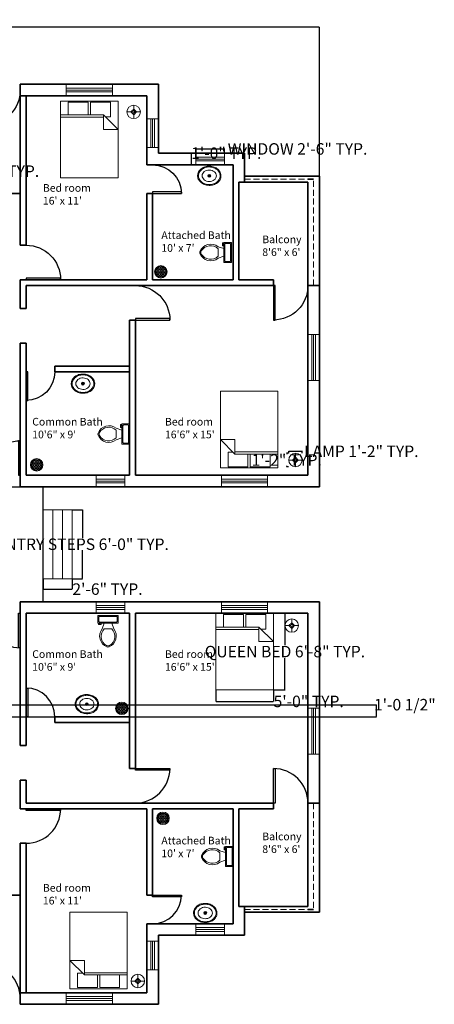
# Model space of a CAD drawing. Units: inches. Extents: x 2450 to 4494, y 1482 to 2597.
# Tile 7 of 7: x 4062 to 4494, y 1559 to 2587. Entities that reach past the tile are written whole.
import ezdxf

# ---------------------------------------------------------------- set-up
doc = ezdxf.new("R2010")
doc.units = ezdxf.units.IN
doc.header["$LTSCALE"] = 5
doc.header["$MEASUREMENT"] = 0
doc.linetypes.add('HIDDEN', pattern=[0.375, 0.25, -0.125])
for name, color, linetype, lineweight in [('A-ANNO-DIMS', 2, 'Continuous', 18), ('A-AREA-IDEN', 7, 'Continuous', 18), ('A-DOOR', 4, 'Continuous', 25), ('A-FLOR-EDGE', 7, 'Continuous', 25), ('A-FLOR-FIXT', 9, 'Continuous', 18), ('A-FLOR-STRS', 7, 'Continuous', 18), ('A-FURN', 8, 'Continuous', 18), ('A-GLAZ', 4, 'Continuous', 18), ('A-WALL', 7, 'Continuous', 35), ('A-WALL-HIDN', 7, 'HIDDEN', 18)]:
    doc.layers.add(name, color=color, linetype=linetype, lineweight=lineweight)
doc.styles.get("Standard").update_dxf_attribs({"font": 'arial.ttf'})
doc.dimstyles.get("Standard").update_dxf_attribs({"dimtxt": 12, "dimasz": 0.18, "dimexe": 0.18, "dimexo": 0.0625, "dimgap": 0.09, "dimtad": 0, "dimtih": 1, "dimtoh": 1, "dimdec": 0, "dimzin": 0, "dimdsep": 46, "dimlunit": 3, "dimtxsty": 'Standard', "dimcen": 0.09, "dimadec": 0, "dimazin": 0, "dimtfac": 1, "dimtdec": 0, "dimtofl": 0, "dimtmove": 0, "dimatfit": 3, "dimfxl": 1, "dimtolj": 1, "dimtzin": 0, "dimarcsym": 0})

# ---------------------------------------------------------------- blocks, each defined once
blk = doc.blocks.new('*U2')
for p, q in [((0, 0), (0, -6)), ((36, 0), (36, -6))]:
    blk.add_line(p, q)
blk.add_lwpolyline([(0, 0), (0, 36), (1.75, 36), (1.75, 0)], close=True)
blk.add_arc((0, 0), 36, 0, 90)
blk = doc.blocks.new('*U3')
for p, q in [((0, 0), (0, -6)), ((30, 0), (30, -6))]:
    blk.add_line(p, q)
blk.add_lwpolyline([(0, 0), (0, 30), (1.75, 30), (1.75, 0)], close=True)
blk.add_arc((0, 0), 30, 0, 90)
blk = doc.blocks.new('*U5')
for p, q in [((-36, 0), (-36, 6)), ((0, 0), (0, 6))]:
    blk.add_line(p, q)
blk.add_lwpolyline([(0, 0), (0, -36), (-1.75, -36), (-1.75, 0)], close=True)
blk.add_arc((0, 0), 36, 180, 270)
blk = doc.blocks.new('Bed - Queen')
for p, q in [((0, -80.00003), (0, 0)), ((0, 0), (59.99999, 0)), ((59.99999, 0), (59.99999, -80.00003)), ((7.99999, -1.2), (28.79998, -1.2)), ((7.99999, -14.4), (7.99999, -1.2)), ((28.79998, -1.2), (28.79998, -14.4)), ((31.19999, -1.2), (51.99999, -1.2)), ((31.19999, -14.4), (31.19999, -1.2)), ((51.99999, -1.2), (51.99999, -16.4)), ((0, -14.4), (44.8, -14.4)), ((44.8, -16.8), (0, -16.8)), ((59.99999, -29.6), (44.8, -14.4)), ((44.8, -14.4), (44.8, -29.6)), ((51.99999, -16.4), (46.79936, -16.4)), ((44.8, -29.6), (59.99999, -29.6)), ((59.99999, -80.00003), (0, -80.00003))]:
    blk.add_line(p, q)
blk = doc.blocks.new('Lamp - Table')
for p, q in [((-1, 0), (-7, 0)), ((0, 3), (-3, 0)), ((-3, 0), (0, -3)), ((0, 7), (0, 1)), ((3, 0), (0, 3)), ((0, -3), (3, 0)), ((1, 0), (7, 0)), ((0, -1), (0, -7))]:
    blk.add_line(p, q)
for radius in [7, 1]:
    blk.add_circle((0, 0), radius)
blk = doc.blocks.new('Toilet - top')
for p, q in [((-10, -8.5), (-8, -8.5)), ((-10, -9.5), (-10, -8.5)), ((-7, -9.5), (-10, -9.5)), ((-8, -8.5), (-8, -8)), ((-7, -8), (-7, -9.5)), ((-4, -8), (-6, -14)), ((4, -8), (6, -14)), ((9.5, -6), (9.5, -2)), ((4, -14), (-4, -14))]:
    blk.add_line(p, q)
blk.add_lwpolyline([(10.5, -8), (10.5, 0), (-10.5, 0), (-10.5, -8)], close=True)
for points in [[(-9.5, -2), (-9.5, -6)], [(8.5, -1), (-8.5, -1)], [(-8.5, -7), (8.5, -7)]]:
    blk.add_lwpolyline(points)
for centre, radius, start, end in [((-8.6, -1.9), 0.884, 81.8699, 188.1301), ((-8.6, -6.1), 0.884, 171.8699, 278.1301), ((8.6, -1.9), 0.884, 351.8699, 98.1301), ((8.6, -6.1), 0.884, 261.8699, 8.1301), ((3.5, -21.6), 12.2, 141.4691, 247.9714), ((4.2, -21.8), 11.3, 136.3677, 238.9468), ((-3.5, -21.6), 12.2, 292.0284, 38.5307), ((-4.2, -21.8), 11.3, 301.053, 43.6321), ((0, -27.9), 4, 245.7318, 294.2682), ((0, -29), 4, 254.8605, 285.1395)]:
    blk.add_arc(centre, radius, start, end)
blk = doc.blocks.new('Sink - Oval top')
for p, q in [((-1, 0), (1, 0)), ((0, 1), (0, -1))]:
    blk.add_line(p, q)
for points in [[(-12.2, 0.4, 0.117634), (-11.5, -3.4, 0.104469), (-8.9, -6.8, 0.090016), (-5.1, -9.1, 0.08192), (-0.3, -10, 0.08192), (4.5, -9.4, 0.090016), (8.4, -7.4, 0.104469), (11.2, -4.1, 0.117634), (12.2, -0.4, 0.117634), (11.5, 3.4, 0.104469), (8.9, 6.8, 0.090016), (5.1, 9.1, 0.08192), (0.3, 10, 0.08192), (-4.5, 9.4, 0.090016), (-8.4, 7.4, 0.104469), (-11.2, 4.1, 0.117634)], [(-11.3, 0.2, 0.118622), (-10.5, -3.3, 0.104678), (-8.1, -6.4, 0.089562), (-4.5, -8.4, 0.081185), (-0.1, -9.2, 0.081185), (4.3, -8.5, 0.089562), (7.9, -6.6, 0.104678), (10.4, -3.5, 0.118622), (11.3, -0.2, 0.118622), (10.5, 3.3, 0.104678), (8.1, 6.4, 0.089562), (4.5, 8.4, 0.081185), (0.1, 9.2, 0.081185), (-4.3, 8.5, 0.089562), (-7.9, 6.6, 0.104678), (-10.4, 3.5, 0.118622)], [(-7.4, 0.1, 0.118283), (-6.9, -2.2, 0.104607), (-5.3, -4.2, 0.089718), (-3, -5.5, 0.081436), (-0.1, -6, 0.081436), (2.8, -5.6, 0.089718), (5.2, -4.3, 0.104607), (6.9, -2.3, 0.118283), (7.4, -0.1, 0.118283), (6.9, 2.2, 0.104607), (5.3, 4.2, 0.089718), (3, 5.5, 0.081436), (0.1, 6, 0.081436), (-2.8, 5.6, 0.089718), (-5.2, 4.3, 0.104607), (-6.9, 2.3, 0.118283)]]:
    blk.add_lwpolyline(points, format="xyb", close=True)
for radius in [1.5, 1]:
    blk.add_circle((0, 0), radius)
blk = doc.blocks.new('WIN-30-FRAME')
for p, q in [((0, 0), (0, 12)), ((0, 12), (30, 12)), ((30, 12), (30, 0)), ((30, 8), (0, 8)), ((30, 6), (0, 6)), ((30, 4), (0, 4)), ((30, 0), (0, 0))]:
    blk.add_line(p, q)
blk = doc.blocks.new('WIN-48-FRAME')
for p, q in [((48, 12), (0, 12)), ((0, 12), (0, 0)), ((48, 0), (48, 12)), ((48, 8), (0, 8)), ((48, 6), (0, 6)), ((48, 4), (0, 4)), ((0, 0), (48, 0))]:
    blk.add_line(p, q)
blk = doc.blocks.new('WIN-30-PART-FRAME')
for p, q in [((12, 30), (0, 30)), ((0, 30), (0, 0)), ((4, 30), (4, 0)), ((6, 30), (6, 0)), ((8, 30), (8, 0)), ((12, 6), (12, 30)), ((0, 0), (12, 0))]:
    blk.add_line(p, q)
blk = doc.blocks.new('WIN-48-PART-FRAME')
for p, q in [((48, 12), (0, 12)), ((0, 12), (0, 0)), ((48, 0), (48, 12)), ((48, 8), (0, 8)), ((48, 6), (0, 6)), ((48, 4), (0, 4)), ((24, 0), (48, 0))]:
    blk.add_line(p, q)
blk = doc.blocks.new('WIN-48-OPEN-SIDE')
for p, q in [((0, 48), (12, 48)), ((4, 48), (4, 0)), ((6, 48), (6, 0)), ((8, 48), (8, 0)), ((12, 48), (12, 0)), ((12, 0), (0, 0))]:
    blk.add_line(p, q)
blk = doc.blocks.new('STEPS-72-ENTRY')
at = {"ltscale": 5}
for p, q in [((0, 72), (30, 72)), ((10, 0), (10, 72)), ((20, 0), (20, 72)), ((30, 0), (30, 72)), ((0, 0), (30, 0))]:
    blk.add_line(p, q, dxfattribs=at)
blk = doc.blocks.new('DRAIN-FLOOR-ROUND')
at = {"ltscale": 5}
h = blk.add_hatch(dxfattribs=at)
h.set_pattern_fill('HONEY', color=256, scale=7)
h.set_pattern_definition([(0, (-4161.689, -1861.538), (1.3125, 0.75777223), [0.875, -1.75]), (120, (-4161.689, -1861.538), (-1.3125, 0.75777223), [0.875, -1.75]), (60, (-4161.689, -1861.538), (3e-16, 1.51554446), [-1.75, 0.875])])
h.paths.add_polyline_path([(1, 6.5, 1), (12, 6.5, 1)])
for radius in [6.52, 5.52]:
    blk.add_circle((6.5, 6.5), radius, dxfattribs=at)
blk = doc.blocks.new('*D39')
at = {"layer": 'A-ANNO-DIMS', "color": 0, "lineweight": -2, "ltscale": 5, "transparency": 16777216}
for p, q in [((4245.3, 2447.3), (4245.3, 2451.9)), ((4245.5, 2451.8), (4275.1, 2451.8)), ((4275.3, 2447.3), (4275.3, 2451.9)), ((4275.3, 2451.8), (4275.5, 2451.8))]:
    blk.add_line(p, q, dxfattribs=at)
at = {"layer": 'A-ANNO-DIMS', "color": 0, "ltscale": 5, "transparency": 16777216}
for points in [[(4245.5, 2451.8), (4245.5, 2451.7), (4245.3, 2451.8)], [(4275.1, 2451.8), (4275.1, 2451.7), (4275.3, 2451.8)]]:
    blk.add_solid(points, dxfattribs=at)
at = {"layer": 'Defpoints', "color": 0, "ltscale": 5, "transparency": 16777216}
for p in [(4245.3, 2447.3), (4275.3, 2451.8), (4275.3, 2447.3)]:
    blk.add_point(p, dxfattribs=at)
at = {"layer": 'A-ANNO-DIMS', "color": 0, "ltscale": 5, "transparency": 16777216, "insert": (4351.5, 2451.8), "char_height": 12, "attachment_point": 5}
blk.add_mtext('\\A1;WINDOW 2\'-6" TYP.', dxfattribs=at)
blk = doc.blocks.new('*D40')
at = {"layer": 'A-ANNO-DIMS', "color": 0, "lineweight": -2, "ltscale": 5, "transparency": 16777216}
for p, q in [((4245.2, 2447.3), (4240.6, 2447.3)), ((4240.8, 2447.3), (4240.8, 2447.4)), ((4240.8, 2447.4), (4241, 2447.4)), ((4240.8, 2435.4), (4240.8, 2447.1)), ((4245.2, 2435.3), (4240.6, 2435.3))]:
    blk.add_line(p, q, dxfattribs=at)
at = {"layer": 'A-ANNO-DIMS', "color": 0, "ltscale": 5, "transparency": 16777216}
for points in [[(4240.8, 2447.1), (4240.8, 2447.1), (4240.8, 2447.3)], [(4240.8, 2435.4), (4240.8, 2435.4), (4240.8, 2435.3)]]:
    blk.add_solid(points, dxfattribs=at)
at = {"layer": 'Defpoints', "color": 0, "ltscale": 5, "transparency": 16777216}
for p in [(4240.8, 2447.3), (4245.3, 2447.3), (4245.3, 2435.3)]:
    blk.add_point(p, dxfattribs=at)
at = {"layer": 'A-ANNO-DIMS', "color": 0, "ltscale": 5, "transparency": 16777216, "insert": (4277.1, 2447.4), "char_height": 12, "attachment_point": 5}
blk.add_mtext('\\A1;1\'-0" TYP.', dxfattribs=at)
blk = doc.blocks.new('*D49')
at = {"layer": 'A-ANNO-DIMS', "color": 0, "lineweight": -2, "ltscale": 5, "transparency": 16777216}
for p, q in [((4326.4, 1967.3), (4338.5, 1967.3)), ((4338.3, 1967.1), (4338.3, 1933.9)), ((4338.3, 1887.4), (4338.3, 1920.6)), ((4326.4, 1887.3), (4338.5, 1887.3))]:
    blk.add_line(p, q, dxfattribs=at)
at = {"layer": 'A-ANNO-DIMS', "color": 0, "ltscale": 5, "transparency": 16777216}
for points in [[(4338.3, 1967.1), (4338.3, 1967.1), (4338.3, 1967.3)], [(4338.3, 1887.4), (4338.3, 1887.4), (4338.3, 1887.3)]]:
    blk.add_solid(points, dxfattribs=at)
at = {"layer": 'Defpoints', "color": 0, "ltscale": 5, "transparency": 16777216}
for p in [(4326.3, 1967.3), (4338.3, 1967.3), (4326.3, 1887.3)]:
    blk.add_point(p, dxfattribs=at)
at = {"layer": 'A-ANNO-DIMS', "color": 0, "ltscale": 5, "transparency": 16777216, "insert": (4338.3, 1927.3), "char_height": 12, "attachment_point": 5}
blk.add_mtext('\\A1;QUEEN BED 6\'-8" TYP.', dxfattribs=at)
blk = doc.blocks.new('*D50')
at = {"layer": 'A-ANNO-DIMS', "color": 0, "lineweight": -2, "ltscale": 5, "transparency": 16777216}
for p, q in [((4266.3, 1887.2), (4266.3, 1875.1)), ((4326.3, 1887.2), (4326.3, 1875.1)), ((4266.5, 1875.3), (4326.1, 1875.3)), ((4326.3, 1875.3), (4326.5, 1875.3))]:
    blk.add_line(p, q, dxfattribs=at)
at = {"layer": 'A-ANNO-DIMS', "color": 0, "ltscale": 5, "transparency": 16777216}
for points in [[(4266.5, 1875.3), (4266.5, 1875.2), (4266.3, 1875.3)], [(4326.1, 1875.3), (4326.1, 1875.2), (4326.3, 1875.3)]]:
    blk.add_solid(points, dxfattribs=at)
at = {"layer": 'Defpoints', "color": 0, "ltscale": 5, "transparency": 16777216}
for p in [(4266.3, 1887.3), (4326.3, 1887.3), (4326.3, 1875.3)]:
    blk.add_point(p, dxfattribs=at)
at = {"layer": 'A-ANNO-DIMS', "color": 0, "ltscale": 5, "transparency": 16777216, "insert": (4363.1, 1875.3), "char_height": 12, "attachment_point": 5}
blk.add_mtext('\\A1;5\'-0" TYP.', dxfattribs=at)
blk = doc.blocks.new('*D51')
at = {"layer": 'A-ANNO-DIMS', "color": 0, "lineweight": -2, "ltscale": 5, "transparency": 16777216}
for p, q in [((4342.3, 2134.2), (4342.3, 2136.5)), ((4342.5, 2136.3), (4356.1, 2136.3)), ((4356.3, 2134.2), (4356.3, 2136.5)), ((4356.3, 2136.3), (4356.5, 2136.3))]:
    blk.add_line(p, q, dxfattribs=at)
at = {"layer": 'A-ANNO-DIMS', "color": 0, "ltscale": 5, "transparency": 16777216}
for points in [[(4342.5, 2136.3), (4342.5, 2136.2), (4342.3, 2136.3)], [(4356.1, 2136.3), (4356.1, 2136.2), (4356.3, 2136.3)]]:
    blk.add_solid(points, dxfattribs=at)
at = {"layer": 'Defpoints', "color": 0, "ltscale": 5, "transparency": 16777216}
for p in [(4342.3, 2134.2), (4356.3, 2136.3), (4356.3, 2134.2)]:
    blk.add_point(p, dxfattribs=at)
at = {"layer": 'A-ANNO-DIMS', "color": 0, "ltscale": 5, "transparency": 16777216, "insert": (4418, 2136.3), "char_height": 12, "attachment_point": 5}
blk.add_mtext('\\A1;LAMP 1\'-2" TYP.', dxfattribs=at)
blk = doc.blocks.new('*D52')
at = {"layer": 'A-ANNO-DIMS', "color": 0, "lineweight": -2, "ltscale": 5, "transparency": 16777216}
for p, q in [((4342.2, 2134.2), (4340, 2134.2)), ((4340.2, 2134), (4340.2, 2133.3)), ((4342.2, 2120.2), (4340, 2120.2)), ((4340.2, 2120.4), (4340.2, 2121.1))]:
    blk.add_line(p, q, dxfattribs=at)
at = {"layer": 'A-ANNO-DIMS', "color": 0, "ltscale": 5, "transparency": 16777216}
for points in [[(4340.1, 2134), (4340.2, 2134), (4340.2, 2134.2)], [(4340.1, 2120.4), (4340.2, 2120.4), (4340.2, 2120.2)]]:
    blk.add_solid(points, dxfattribs=at)
at = {"layer": 'Defpoints', "color": 0, "ltscale": 5, "transparency": 16777216}
for p in [(4340.2, 2134.2), (4342.3, 2134.2), (4342.3, 2120.2)]:
    blk.add_point(p, dxfattribs=at)
at = {"layer": 'A-ANNO-DIMS', "color": 0, "ltscale": 5, "transparency": 16777216, "insert": (4340.2, 2127.2), "char_height": 12, "attachment_point": 5}
blk.add_mtext('\\A1;1\'-2" TYP.', dxfattribs=at)
blk = doc.blocks.new('*D65')
at = {"layer": 'A-ANNO-DIMS', "color": 0, "lineweight": -2, "ltscale": 5, "transparency": 16777216}
for p, q in [((4014, 2458.6), (4023.1, 2458.6)), ((4022.9, 2458.4), (4022.9, 2434.9)), ((4022.9, 2398.7), (4022.9, 2422.3)), ((4014, 2398.6), (4023.1, 2398.6))]:
    blk.add_line(p, q, dxfattribs=at)
at = {"layer": 'A-ANNO-DIMS', "color": 0, "ltscale": 5, "transparency": 16777216}
for points in [[(4022.9, 2458.4), (4022.9, 2458.4), (4022.9, 2458.6)], [(4022.9, 2398.7), (4022.9, 2398.7), (4022.9, 2398.6)]]:
    blk.add_solid(points, dxfattribs=at)
at = {"layer": 'Defpoints', "color": 0, "ltscale": 5, "transparency": 16777216}
for p in [(4013.9, 2458.6), (4022.9, 2458.6), (4013.9, 2398.6)]:
    blk.add_point(p, dxfattribs=at)
at = {"layer": 'A-ANNO-DIMS', "color": 0, "ltscale": 5, "transparency": 16777216, "insert": (4022.9, 2428.6), "char_height": 12, "attachment_point": 5}
blk.add_mtext('\\A1;DESK 5\'-0" TYP.', dxfattribs=at)
blk = doc.blocks.new('*D67')
at = {"layer": 'A-ANNO-DIMS', "color": 0, "lineweight": -2, "ltscale": 5, "transparency": 16777216}
for p, q in [((4116.4, 2075.3), (4127.3, 2075.3)), ((4127.1, 2075.1), (4127.1, 2045.6)), ((4127.1, 2003.4), (4127.1, 2033)), ((4116.4, 2003.3), (4127.3, 2003.3))]:
    blk.add_line(p, q, dxfattribs=at)
at = {"layer": 'A-ANNO-DIMS', "color": 0, "ltscale": 5, "transparency": 16777216}
for points in [[(4127.1, 2075.1), (4127.1, 2075.1), (4127.1, 2075.3)], [(4127.1, 2003.4), (4127.1, 2003.4), (4127.1, 2003.3)]]:
    blk.add_solid(points, dxfattribs=at)
at = {"layer": 'Defpoints', "color": 0, "ltscale": 5, "transparency": 16777216}
for p in [(4116.3, 2075.3), (4127.1, 2075.3), (4116.3, 2003.3)]:
    blk.add_point(p, dxfattribs=at)
at = {"layer": 'A-ANNO-DIMS', "color": 0, "ltscale": 5, "transparency": 16777216, "insert": (4127.1, 2039.3), "char_height": 12, "attachment_point": 5}
blk.add_mtext('\\A1;ENTRY STEPS 6\'-0" TYP.', dxfattribs=at)
blk = doc.blocks.new('*D68')
at = {"layer": 'A-ANNO-DIMS', "color": 0, "lineweight": -2, "ltscale": 5, "transparency": 16777216}
for p, q in [((4086.3, 2003.2), (4086.3, 1992.3)), ((4116.3, 2003.2), (4116.3, 1992.3)), ((4086.5, 1992.5), (4116.1, 1992.5)), ((4116.3, 1992.5), (4116.5, 1992.5))]:
    blk.add_line(p, q, dxfattribs=at)
at = {"layer": 'A-ANNO-DIMS', "color": 0, "ltscale": 5, "transparency": 16777216}
for points in [[(4086.5, 1992.5), (4086.5, 1992.4), (4086.3, 1992.5)], [(4116.1, 1992.5), (4116.1, 1992.4), (4116.3, 1992.5)]]:
    blk.add_solid(points, dxfattribs=at)
at = {"layer": 'Defpoints', "color": 0, "ltscale": 5, "transparency": 16777216}
for p in [(4086.3, 2003.3), (4116.3, 2003.3), (4116.3, 1992.5)]:
    blk.add_point(p, dxfattribs=at)
at = {"layer": 'A-ANNO-DIMS', "color": 0, "ltscale": 5, "transparency": 16777216, "insert": (4153.2, 1992.5), "char_height": 12, "attachment_point": 5}
blk.add_mtext('\\A1;2\'-6" TYP.', dxfattribs=at)
blk = doc.blocks.new('*D71')
at = {"layer": 'A-ANNO-DIMS', "color": 0, "lineweight": -2, "ltscale": 5, "transparency": 16777216}
for p, q in [((3258.3, 2423.3), (3258.3, 2578.9)), ((3258.5, 2578.8), (3795.6, 2578.8)), ((4374.1, 2578.8), (3837, 2578.8)), ((4374.3, 2423.3), (4374.3, 2578.9))]:
    blk.add_line(p, q, dxfattribs=at)
at = {"layer": 'A-ANNO-DIMS', "color": 0, "ltscale": 5, "transparency": 16777216}
for points in [[(3258.5, 2578.8), (3258.5, 2578.7), (3258.3, 2578.8)], [(4374.1, 2578.8), (4374.1, 2578.7), (4374.3, 2578.8)]]:
    blk.add_solid(points, dxfattribs=at)
at = {"layer": 'Defpoints', "color": 0, "ltscale": 5, "transparency": 16777216}
for p in [(4374.3, 2578.8), (3258.3, 2423.3), (4374.3, 2423.3)]:
    blk.add_point(p, dxfattribs=at)
at = {"layer": 'A-ANNO-DIMS', "color": 0, "ltscale": 5, "transparency": 16777216, "insert": (3816.3, 2578.8), "char_height": 12, "attachment_point": 5}
blk.add_mtext('\\A1;93\'-0"', dxfattribs=at)
blk = doc.blocks.new('*D87')
at = {"layer": 'A-ANNO-DIMS', "color": 0, "lineweight": -2, "ltscale": 5, "transparency": 16777216}
for p, q in [((3504.9, 1871.8), (4434, 1871.8)), ((4433.8, 1871.8), (4433.8, 1871.9)), ((4433.8, 1871.9), (4434, 1871.9)), ((4433.8, 1859.4), (4433.8, 1871.6)), ((3534.4, 1859.3), (4434, 1859.3))]:
    blk.add_line(p, q, dxfattribs=at)
at = {"layer": 'A-ANNO-DIMS', "color": 0, "ltscale": 5, "transparency": 16777216}
for points in [[(4433.8, 1871.6), (4433.8, 1871.6), (4433.8, 1871.8)], [(4433.8, 1859.4), (4433.8, 1859.4), (4433.8, 1859.3)]]:
    blk.add_solid(points, dxfattribs=at)
at = {"layer": 'Defpoints', "color": 0, "ltscale": 5, "transparency": 16777216}
for p in [(3504.9, 1871.8), (4433.8, 1871.8), (3534.3, 1859.3)]:
    blk.add_point(p, dxfattribs=at)
at = {"layer": 'A-ANNO-DIMS', "color": 0, "ltscale": 5, "transparency": 16777216, "insert": (4463.4, 1871.9), "char_height": 12, "attachment_point": 5}
blk.add_mtext('\\A1;1\'-0 1/2"', dxfattribs=at)

msp = doc.modelspace()

# ---------------------------------------------------------------- linework, layer by layer
at = {"layer": 'A-FLOR-EDGE', "ltscale": 5}
for p in [(3546.29, 2099.27), (4086.29, 1979.27)]:
    msp.add_line(p, (4086.29, 2099.27), dxfattribs=at)
at = {"layer": 'A-WALL'}
for p, q in [((4062.29, 2519.27), (4206.29, 2519.27)), ((4062.29, 2507.27), (4062.29, 2519.27)), ((4206.29, 2507.27), (4206.29, 2519.27)), ((4062.29, 2507.27), (4194.29, 2507.27)), ((4062.29, 2351.27), (4062.29, 2507.27)), ((4068.29, 2351.27), (4068.29, 2507.27)), ((4194.29, 2507.27), (4194.29, 2435.27)), ((4206.29, 2507.27), (4206.29, 2447.27)), ((4284.29, 2447.27), (4206.29, 2447.27)), ((4284.29, 2447.27), (4296.29, 2447.27)), ((4296.29, 2447.27), (4296.29, 2423.27)), ((4200.29, 2435.27), (4194.29, 2435.27)), ((4284.29, 2435.27), (4200.29, 2435.27)), ((4284.29, 2435.27), (4284.29, 2315.27)), ((4290.29, 2417.27), (4290.29, 2315.27)), ((4362.29, 2417.27), (4290.29, 2417.27)), ((4362.29, 2423.27), (4296.29, 2423.27)), ((4296.29, 2423.27), (4296.29, 2417.27)), ((4362.29, 2423.27), (4374.29, 2423.27)), ((4362.29, 2420.27), (4368.29, 2420.27)), ((4362.29, 2417.27), (4362.29, 2315.27)), ((4374.29, 2423.27), (4374.29, 2099.27)), ((4062.29, 2405.27), (3930.29, 2405.27)), ((4194.29, 2405.27), (4194.29, 2315.27)), ((4200.29, 2405.27), (4194.29, 2405.27)), ((4200.29, 2405.27), (4200.29, 2315.27)), ((4068.29, 2351.27), (4062.29, 2351.27)), ((4062.29, 2285.27), (4062.29, 2315.27)), ((4068.29, 2315.27), (4062.29, 2315.27)), ((4176.29, 2315.27), (4068.29, 2315.27)), ((4182.29, 2315.27), (4176.29, 2315.27)), ((4194.29, 2315.27), (4182.29, 2315.27)), ((4284.29, 2315.27), (4200.29, 2315.27)), ((4326.29, 2315.27), (4290.29, 2315.27)), ((4326.29, 2309.27), (4326.29, 2315.27)), ((4362.29, 2309.27), (4362.29, 2315.27)), ((4068.29, 2285.27), (4068.29, 2309.27)), ((4176.29, 2309.27), (4068.29, 2309.27)), ((4176.29, 2309.27), (4182.29, 2309.27)), ((4326.29, 2309.27), (4182.29, 2309.27)), ((4362.29, 2309.27), (4362.29, 2111.27)), ((4362.29, 2309.27), (4374.29, 2309.27)), ((4068.29, 2285.27), (4062.29, 2285.27)), ((4176.29, 2111.27), (4176.29, 2273.27)), ((4176.29, 2273.27), (4182.29, 2273.27)), ((4182.29, 2111.27), (4182.29, 2273.27)), ((4062.29, 2111.27), (4062.29, 2249.27)), ((4068.29, 2249.27), (4062.29, 2249.27)), ((4068.29, 2225.27), (4068.29, 2249.27)), ((4068.29, 2219.27), (4068.29, 2225.27)), ((4068.29, 2111.27), (4068.29, 2219.27)), ((4176.29, 2225.27), (4098.29, 2225.27)), ((4098.29, 2219.27), (4098.29, 2225.27)), ((4176.29, 2219.27), (4098.29, 2219.27)), ((4062.29, 2111.27), (4062.29, 2099.27)), ((4176.29, 2111.27), (4068.29, 2111.27)), ((4362.29, 2111.27), (4182.29, 2111.27)), ((4374.29, 2099.27), (4062.29, 2099.27)), ((4374.29, 1979.27), (4062.29, 1979.27)), ((4062.29, 1967.27), (4062.29, 1979.27)), ((4374.29, 1655.27), (4374.29, 1979.27)), ((4062.29, 1967.27), (4062.29, 1829.27)), ((4176.29, 1967.27), (4068.29, 1967.27)), ((4068.29, 1967.27), (4068.29, 1859.27)), ((4176.29, 1967.27), (4176.29, 1805.27)), ((4362.29, 1967.27), (4182.29, 1967.27)), ((4182.29, 1967.27), (4182.29, 1805.27)), ((4362.29, 1769.27), (4362.29, 1967.27)), ((4068.29, 1859.27), (4068.29, 1853.27)), ((4068.29, 1853.27), (4068.29, 1829.27)), ((4176.29, 1859.27), (4098.29, 1859.27)), ((4098.29, 1859.27), (4098.29, 1853.27)), ((4176.29, 1853.27), (4098.29, 1853.27)), ((4068.29, 1829.27), (4062.29, 1829.27)), ((4176.29, 1805.27), (4182.29, 1805.27)), ((4062.29, 1793.27), (4062.29, 1763.27)), ((4068.29, 1793.27), (4062.29, 1793.27)), ((4068.29, 1793.27), (4068.29, 1769.27)), ((4176.29, 1769.27), (4068.29, 1769.27)), ((4176.29, 1769.27), (4182.29, 1769.27)), ((4326.29, 1769.27), (4182.29, 1769.27)), ((4326.29, 1769.27), (4326.29, 1763.27)), ((4362.29, 1769.27), (4362.29, 1763.27)), ((4362.29, 1769.27), (4374.29, 1769.27)), ((4068.29, 1763.27), (4062.29, 1763.27)), ((4176.29, 1763.27), (4068.29, 1763.27)), ((4182.29, 1763.27), (4176.29, 1763.27)), ((4194.29, 1763.27), (4182.29, 1763.27)), ((4194.29, 1673.27), (4194.29, 1763.27)), ((4200.29, 1673.27), (4200.29, 1763.27)), ((4284.29, 1763.27), (4200.29, 1763.27)), ((4284.29, 1643.27), (4284.29, 1763.27)), ((4290.29, 1661.27), (4290.29, 1763.27)), ((4326.29, 1763.27), (4290.29, 1763.27)), ((4362.29, 1661.27), (4362.29, 1763.27)), ((4062.29, 1727.27), (4062.29, 1571.27)), ((4068.29, 1727.27), (4062.29, 1727.27)), ((4068.29, 1727.27), (4068.29, 1571.27)), ((4062.29, 1673.27), (3930.29, 1673.27)), ((4200.29, 1673.27), (4194.29, 1673.27)), ((4362.29, 1661.27), (4290.29, 1661.27)), ((4296.29, 1655.27), (4296.29, 1661.27)), ((4296.29, 1631.27), (4296.29, 1655.27)), ((4362.29, 1655.27), (4296.29, 1655.27)), ((4362.29, 1658.27), (4368.29, 1658.27)), ((4362.29, 1655.27), (4374.29, 1655.27)), ((4194.29, 1571.27), (4194.29, 1643.27)), ((4200.29, 1643.27), (4194.29, 1643.27)), ((4284.29, 1643.27), (4200.29, 1643.27)), ((4206.29, 1571.27), (4206.29, 1631.27)), ((4284.29, 1631.27), (4206.29, 1631.27)), ((4284.29, 1631.27), (4296.29, 1631.27)), ((4062.29, 1571.27), (4194.29, 1571.27)), ((4062.29, 1571.27), (4062.29, 1559.27)), ((4206.29, 1571.27), (4206.29, 1559.27)), ((4062.29, 1559.27), (4206.29, 1559.27))]:
    msp.add_line(p, q, dxfattribs=at)
at = {"layer": 'A-WALL-HIDN', "ltscale": 5}
for p, q in [((4296.29, 2420.27), (4362.29, 2420.27)), ((4368.29, 2309.27), (4368.29, 2420.27)), ((4368.29, 1769.27), (4368.29, 1658.27)), ((4296.29, 1658.27), (4362.29, 1658.27))]:
    msp.add_line(p, q, dxfattribs=at)

# ---------------------------------------------------------------- block references
at = {"layer": 'A-DOOR', "xscale": -1}
for name, p, rotation in [('*U2', (4026.29, 2513.27), 180), ('*U3', (4200.29, 2405.27), 270), ('*U2', (4068.29, 2315.27), 270), ('*U2', (4326.29, 2309.27), 180), ('*U2', (4182.29, 2273.27), 270), ('*U3', (4068.29, 2219.27), 180), ('*U5', (4062.29, 2111.27), 180)]:
    msp.add_blockref(name, p, dxfattribs=dict(at, rotation=rotation))
at = {"layer": 'A-DOOR'}
for name, p in [('*U5', (4062.29, 1967.27)), ('*U3', (4068.29, 1859.27)), ('*U2', (4326.29, 1769.27)), ('*U2', (4026.29, 1565.27))]:
    msp.add_blockref(name, p, dxfattribs=at)
at = {"layer": 'A-DOOR', "rotation": 270}
for name, p in [('*U2', (4182.29, 1805.27)), ('*U2', (4068.29, 1763.27)), ('*U3', (4200.29, 1673.27))]:
    msp.add_blockref(name, p, dxfattribs=at)
at = {"layer": 'A-FLOR-FIXT', "ltscale": 5}
for name, p in [('Sink - Oval top', (4259.42, 2423.78)), ('Sink - Oval top', (4127.66, 2206.86)), ('Toilet - top', (4153.74, 1965.04)), ('Sink - Oval top', (4131.67, 1872.48)), ('Sink - Oval top', (4255.21, 1654.55))]:
    msp.add_blockref(name, p, dxfattribs=at)
at = {"layer": 'A-FLOR-FIXT', "ltscale": 5, "rotation": 270}
for p in [(4282.56, 2343.73), (4176.29, 2154.29), (4284.29, 1713.5)]:
    msp.add_blockref('Toilet - top', p, dxfattribs=at)
at = {"layer": 'A-FLOR-FIXT'}
for p in [(4202.4, 2317.09), (4072.85, 2115.65), (4161.69, 1861.54), (4204.55, 1746.86)]:
    msp.add_blockref('DRAIN-FLOOR-ROUND', p, dxfattribs=at)
at = {"layer": 'A-FLOR-STRS'}
msp.add_blockref('STEPS-72-ENTRY', (4086.29, 2003.27), dxfattribs=at)
at = {"layer": 'A-FURN', "ltscale": 5}
for name, p in [('Bed - Queen', (4104.29, 2501.8)), ('Lamp - Table', (4180.56, 2490.38)), ('Lamp - Table', (4349.28, 2127.17)), ('Bed - Queen', (4266.29, 1967.27)), ('Lamp - Table', (4345.48, 1954.43)), ('Lamp - Table', (4184.87, 1583.58))]:
    msp.add_blockref(name, p, dxfattribs=at)
at = {"layer": 'A-FURN', "ltscale": 5, "rotation": 180}
for p in [(4330.95, 2118.9), (4173.91, 1575.47)]:
    msp.add_blockref('Bed - Queen', p, dxfattribs=at)
at = {"layer": 'A-GLAZ', "extrusion": (0, 0, -1), "zscale": -1, "rotation": 180}
for name, p in [('WIN-48-PART-FRAME', (-4110.29, 2519.27)), ('WIN-30-PART-FRAME', (-4194.29, 2483.27))]:
    msp.add_blockref(name, p, dxfattribs=at)
at = {"layer": 'A-GLAZ'}
for name, p in [('WIN-30-FRAME', (4245.29, 2435.27)), ('WIN-48-OPEN-SIDE', (4362.29, 2210.27)), ('WIN-48-FRAME', (4272.29, 2099.27)), ('WIN-48-OPEN-SIDE', (4362.29, 1820.27)), ('WIN-30-PART-FRAME', (4194.29, 1595.27)), ('WIN-48-PART-FRAME', (4110.29, 1559.27))]:
    msp.add_blockref(name, p, dxfattribs=at)
at = {"layer": 'A-GLAZ', "rotation": 180}
for name, p in [('WIN-30-FRAME', (4171.28, 2111.27)), ('WIN-30-FRAME', (4171.28, 1979.27)), ('WIN-48-FRAME', (4320.29, 1979.27)), ('WIN-30-FRAME', (4275.29, 1643.27))]:
    msp.add_blockref(name, p, dxfattribs=at)

# ---------------------------------------------------------------- texts
at = {"layer": 'A-AREA-IDEN', "char_height": 8}
for s, insert, attachment_point in [("Bed room\\P16' x 11'", (4085.86, 2393.76), 7), ("Attached Bath\\P10' x 7'", (4209.43, 2344.44), 7), ('Balcony\\P8\'6" x 6\'', (4314.69, 2340.08), 7), ('Common Bath\\P10\'6" x 9\'', (4074.72, 2149.83), 7), ('Bed room\\P16\'6" x 15\'', (4213.19, 2149.83), 7), ('Common Bath\\P10\'6" x 9\'', (4074.72, 1928.7), 1), ('Bed room\\P16\'6" x 15\'', (4213.19, 1928.7), 1), ('Balcony\\P8\'6" x 6\'', (4314.69, 1738.45), 1), ("Attached Bath\\P10' x 7'", (4209.43, 1734.1), 1), ("Bed room\\P16' x 11'", (4085.86, 1684.77), 1)]:
    msp.add_mtext_dynamic_manual_height_columns(s, width=155.5618, gutter_width=1, heights=[0], dxfattribs=dict(at, insert=insert, attachment_point=attachment_point))

# ---------------------------------------------------------------- dimensions: what is measured, and where the dimension line sits
at = {"layer": 'A-ANNO-DIMS', "ltscale": 5}
dim = msp.add_linear_dim(base=(4374.29, 2578.77), p1=(3258.29, 2423.27), p2=(4374.29, 2423.27), dimstyle='Standard', override={"dimdec": 1, "dimlfac": 1, "dimrnd": 0, "dimzin": 1, "dimdsep": 46, "dimlunit": 4, "dimfrac": 2}, dxfattribs=at)
dim.commit()
dim.dimension.update_dxf_attribs({"geometry": '*D71', "text_midpoint": (3816.29, 2578.77)})
for base, p1, p2, text, picture, middle in [((4275.29, 2451.77), (4245.29, 2447.27), (4275.29, 2447.27), 'WINDOW <> TYP.', '*D39', (4351.48, 2451.77)), ((4356.28, 2136.27), (4342.28, 2134.17), (4356.28, 2134.17), 'LAMP <> TYP.', '*D51', (4418.01, 2136.27)), ((4116.29, 1992.47), (4086.29, 2003.27), (4116.29, 2003.27), '<> TYP.', '*D68', (4153.24, 1992.47)), ((4326.29, 1875.27), (4266.29, 1887.27), (4326.29, 1887.27), '<> TYP.', '*D50', (4363.13, 1875.27))]:
    dim = msp.add_linear_dim(base=base, p1=p1, p2=p2, text=text, dimstyle='Standard', override={"dimdec": 1, "dimlfac": 1, "dimrnd": 0, "dimzin": 1, "dimdsep": 46, "dimlunit": 4, "dimfrac": 2}, dxfattribs=at)
    dim.commit()
    dim.dimension.update_dxf_attribs({"geometry": picture, "text_midpoint": middle})
for base, p1, p2, text, picture, middle in [((4022.89, 2458.56), (4013.89, 2398.56), (4013.89, 2458.56), 'DESK <> TYP.', '*D65', (4022.89, 2428.56)), ((4240.79, 2447.27), (4245.29, 2435.27), (4245.29, 2447.27), '<> TYP.', '*D40', (4277.07, 2447.45)), ((4340.18, 2134.17), (4342.28, 2120.17), (4342.28, 2134.17), '<> TYP.', '*D52', (4340.18, 2127.17)), ((4127.09, 2075.27), (4116.29, 2003.27), (4116.29, 2075.27), 'ENTRY STEPS <> TYP.', '*D67', (4127.09, 2039.27)), ((4338.29, 1967.27), (4326.29, 1887.27), (4326.29, 1967.27), 'QUEEN BED <> TYP.', '*D49', (4338.29, 1927.27))]:
    dim = msp.add_linear_dim(base=base, p1=p1, p2=p2, angle=90, text=text, dimstyle='Standard', override={"dimdec": 1, "dimlfac": 1, "dimrnd": 0, "dimzin": 1, "dimdsep": 46, "dimlunit": 4, "dimfrac": 2}, dxfattribs=at)
    dim.commit()
    dim.dimension.update_dxf_attribs({"geometry": picture, "text_midpoint": middle})
dim = msp.add_linear_dim(base=(4433.79, 1871.76), p1=(3534.29, 1859.27), p2=(3504.89, 1871.76), angle=90, dimstyle='Standard', override={"dimdec": 1, "dimlfac": 1, "dimrnd": 0, "dimzin": 1, "dimdsep": 46, "dimlunit": 4, "dimfrac": 2}, dxfattribs=at)
dim.commit()
dim.dimension.update_dxf_attribs({"geometry": '*D87', "text_midpoint": (4463.43, 1871.94)})

doc.saveas('drawing.dxf')
